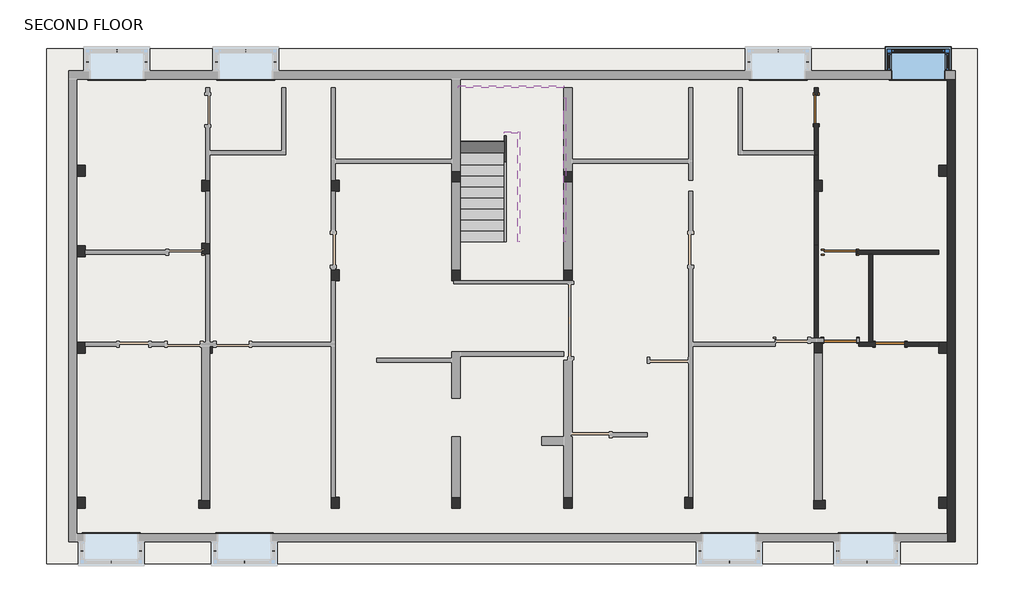
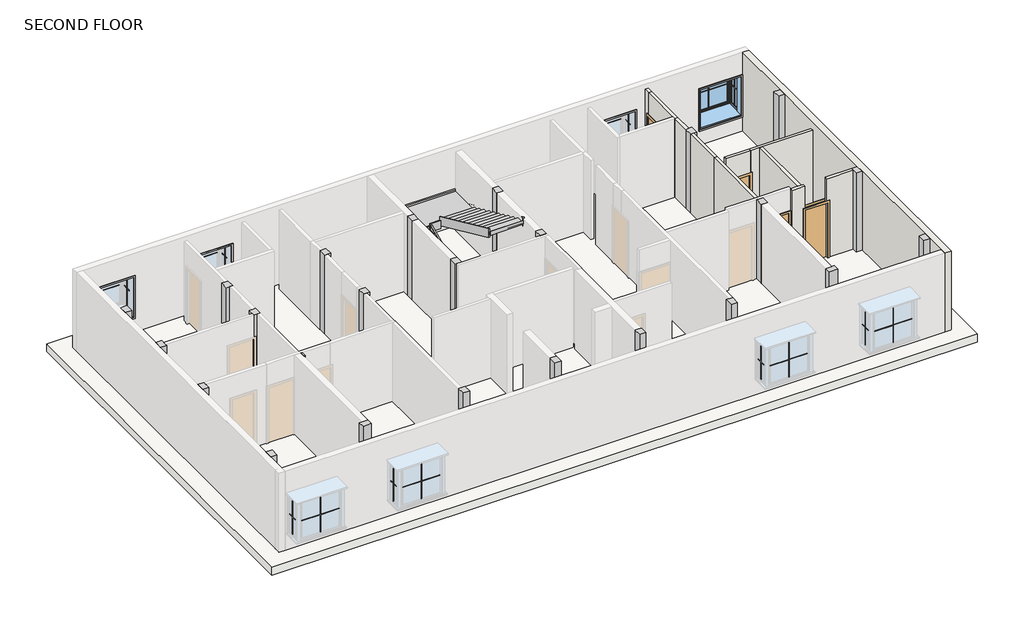
# One storey, part 2 of 2: 32 proxies, 24 columns, 11 walls, 6 members, 4 doors, 1 slab, 1 stair flight, 1 window.
"""IFC4 building model written with IfcOpenShell, lengths in millimetres."""

from ifc_helpers import new_model, si_unit, frame, origin, place, context, project, spatial, polyline, outline, extrude, faceted_brep, transform, mapped, element, save
from components import m_muntin_pattern_2x2_m_muntin_pattern_2x2_c1fd4460, m_muntin_pattern_2x2_m_muntin_pattern_2x2_777b163a, m_trim_window_interior_flat_picture_frame_44e8afef, column_216859a2, door_1991e9a2, door_a431d384, door_82def9da, m_door_single_panel_3_x7_f8176753, stair_flight_b17f4745, window_19bbd869

model = new_model("IFC4")

# Units and contexts
model_context = context("Model", 3, world=origin())
ifc_project = project(units=[si_unit("LENGTHUNIT", "METRE", prefix="MILLI")], contexts=[model_context])

# Site, building, storey
site = spatial("IfcSite", under=ifc_project)
building = spatial("IfcBuilding", under=site)
storey = spatial("IfcBuildingStorey", under=building, Name="SECOND FLOOR", Elevation=9601.2)

# Proxies
placement = place(None, origin())
m_muntin_pattern_2x2_m_muntin_pattern_2x2_shape = m_muntin_pattern_2x2_m_muntin_pattern_2x2_c1fd4460(model_context)
element("IfcBuildingElementProxy", 1, Name="M_Muntin Pattern_2x2 : M_Muntin Pattern_2x2", ObjectType="M_Muntin Pattern_2x2 : M_Muntin Pattern_2x2", at=placement, inside=storey, context=model_context, shape_type="MappedRepresentation", body=[
    mapped(m_muntin_pattern_2x2_m_muntin_pattern_2x2_shape, transform((-11500.7987957, -5499.9182661, 10321.85), x_axis=(-1.0, 0.0, 0.0), y_axis=(0.0, -1.0, 0.0), z_axis=(0.0, 0.0, 1.0))),
])
element("IfcBuildingElementProxy", 2, Name="M_Muntin Pattern_2x2 : M_Muntin Pattern_2x2", ObjectType="M_Muntin Pattern_2x2 : M_Muntin Pattern_2x2", at=placement, inside=storey, context=model_context, shape_type="MappedRepresentation", body=[
    mapped(m_muntin_pattern_2x2_m_muntin_pattern_2x2_shape, transform((-7819.250543, -5499.9182661, 10321.85), x_axis=(-1.0, 0.0, 0.0), y_axis=(0.0, -1.0, 0.0), z_axis=(0.0, 0.0, 1.0))),
])
element("IfcBuildingElementProxy", 3, Name="M_Muntin Pattern_2x2 : M_Muntin Pattern_2x2", ObjectType="M_Muntin Pattern_2x2 : M_Muntin Pattern_2x2", at=placement, inside=storey, context=model_context, shape_type="MappedRepresentation", body=[
    mapped(m_muntin_pattern_2x2_m_muntin_pattern_2x2_shape, transform((5599.7512082, -5499.9182661, 10321.85), x_axis=(-1.0, 0.0, 0.0), y_axis=(0.0, -1.0, 0.0), z_axis=(0.0, 0.0, 1.0))),
])
element("IfcBuildingElementProxy", 4, Name="M_Muntin Pattern_2x2 : M_Muntin Pattern_2x2", ObjectType="M_Muntin Pattern_2x2 : M_Muntin Pattern_2x2", at=placement, inside=storey, context=model_context, shape_type="MappedRepresentation", body=[
    mapped(m_muntin_pattern_2x2_m_muntin_pattern_2x2_shape, transform((9408.6146942, -5499.9182662, 10321.85), x_axis=(-1.0, 0.0, 0.0), y_axis=(0.0, -1.0, 0.0), z_axis=(0.0, 0.0, 1.0))),
])
element("IfcBuildingElementProxy", 5, Name="M_Muntin Pattern_2x2 : M_Muntin Pattern_2x2", ObjectType="M_Muntin Pattern_2x2 : M_Muntin Pattern_2x2", at=placement, inside=storey, context=model_context, shape_type="MappedRepresentation", body=[
    mapped(m_muntin_pattern_2x2_m_muntin_pattern_2x2_shape, transform((-11348.3987957, 8647.7317329, 10321.85), x_axis=(1.0, 0.0, 0.0), y_axis=(0.0, 1.0, 0.0), z_axis=(0.0, 0.0, 1.0))),
])
element("IfcBuildingElementProxy", 6, Name="M_Muntin Pattern_2x2 : M_Muntin Pattern_2x2", ObjectType="M_Muntin Pattern_2x2 : M_Muntin Pattern_2x2", at=placement, inside=storey, context=model_context, shape_type="MappedRepresentation", body=[
    mapped(m_muntin_pattern_2x2_m_muntin_pattern_2x2_shape, transform((-7779.6987993, 8647.7317329, 10321.85), x_axis=(1.0, 0.0, 0.0), y_axis=(0.0, 1.0, 0.0), z_axis=(0.0, 0.0, 1.0))),
])
element("IfcBuildingElementProxy", 7, Name="M_Muntin Pattern_2x2 : M_Muntin Pattern_2x2", ObjectType="M_Muntin Pattern_2x2 : M_Muntin Pattern_2x2", at=placement, inside=storey, context=model_context, shape_type="MappedRepresentation", body=[
    mapped(m_muntin_pattern_2x2_m_muntin_pattern_2x2_shape, transform((6952.301208, 8647.7317329, 10321.85), x_axis=(1.0, 0.0, 0.0), y_axis=(0.0, 1.0, 0.0), z_axis=(0.0, 0.0, 1.0))),
])
element("IfcBuildingElementProxy", 8, Name="M_Muntin Pattern_2x2 : M_Muntin Pattern_2x2", ObjectType="M_Muntin Pattern_2x2 : M_Muntin Pattern_2x2", at=placement, inside=storey, context=model_context, shape_type="MappedRepresentation", body=[
    mapped(m_muntin_pattern_2x2_m_muntin_pattern_2x2_shape, transform((10825.8012075, 8647.7317329, 10321.85), x_axis=(1.0, 0.0, 0.0), y_axis=(0.0, 1.0, 0.0), z_axis=(0.0, 0.0, 1.0))),
])
m_muntin_pattern_2x2_m_muntin_pattern_2x2_2_shape = m_muntin_pattern_2x2_m_muntin_pattern_2x2_777b163a(model_context)
element("IfcBuildingElementProxy", 9, Name="M_Muntin Pattern_2x2 : M_Muntin Pattern_2x2", ObjectType="M_Muntin Pattern_2x2 : M_Muntin Pattern_2x2", at=placement, inside=storey, context=model_context, shape_type="MappedRepresentation", body=[
    mapped(m_muntin_pattern_2x2_m_muntin_pattern_2x2_2_shape, transform((-10690.4737957, -5190.3932661, 10321.85), x_axis=(0.0, 1.0, 0.0), y_axis=(-1.0, 0.0, 0.0), z_axis=(0.0, 0.0, 1.0))),
])
element("IfcBuildingElementProxy", 10, Name="M_Muntin Pattern_2x2 : M_Muntin Pattern_2x2", ObjectType="M_Muntin Pattern_2x2 : M_Muntin Pattern_2x2", at=placement, inside=storey, context=model_context, shape_type="MappedRepresentation", body=[
    mapped(m_muntin_pattern_2x2_m_muntin_pattern_2x2_2_shape, transform((-12311.1237957, -5190.3932661, 10321.85), x_axis=(0.0, -1.0, 0.0), y_axis=(1.0, 0.0, 0.0), z_axis=(0.0, 0.0, 1.0))),
])
element("IfcBuildingElementProxy", 11, Name="M_Muntin Pattern_2x2 : M_Muntin Pattern_2x2", ObjectType="M_Muntin Pattern_2x2 : M_Muntin Pattern_2x2", at=placement, inside=storey, context=model_context, shape_type="MappedRepresentation", body=[
    mapped(m_muntin_pattern_2x2_m_muntin_pattern_2x2_2_shape, transform((-7008.925543, -5190.3932661, 10321.85), x_axis=(0.0, 1.0, 0.0), y_axis=(-1.0, 0.0, 0.0), z_axis=(0.0, 0.0, 1.0))),
])
element("IfcBuildingElementProxy", 12, Name="M_Muntin Pattern_2x2 : M_Muntin Pattern_2x2", ObjectType="M_Muntin Pattern_2x2 : M_Muntin Pattern_2x2", at=placement, inside=storey, context=model_context, shape_type="MappedRepresentation", body=[
    mapped(m_muntin_pattern_2x2_m_muntin_pattern_2x2_2_shape, transform((-8629.575543, -5190.3932661, 10321.85), x_axis=(0.0, -1.0, 0.0), y_axis=(1.0, 0.0, 0.0), z_axis=(0.0, 0.0, 1.0))),
])
element("IfcBuildingElementProxy", 13, Name="M_Muntin Pattern_2x2 : M_Muntin Pattern_2x2", ObjectType="M_Muntin Pattern_2x2 : M_Muntin Pattern_2x2", at=placement, inside=storey, context=model_context, shape_type="MappedRepresentation", body=[
    mapped(m_muntin_pattern_2x2_m_muntin_pattern_2x2_2_shape, transform((6410.0762082, -5190.3932661, 10321.85), x_axis=(0.0, 1.0, 0.0), y_axis=(-1.0, 0.0, 0.0), z_axis=(0.0, 0.0, 1.0))),
])
element("IfcBuildingElementProxy", 14, Name="M_Muntin Pattern_2x2 : M_Muntin Pattern_2x2", ObjectType="M_Muntin Pattern_2x2 : M_Muntin Pattern_2x2", at=placement, inside=storey, context=model_context, shape_type="MappedRepresentation", body=[
    mapped(m_muntin_pattern_2x2_m_muntin_pattern_2x2_2_shape, transform((4789.4262082, -5190.3932661, 10321.85), x_axis=(0.0, -1.0, 0.0), y_axis=(1.0, 0.0, 0.0), z_axis=(0.0, 0.0, 1.0))),
])
element("IfcBuildingElementProxy", 15, Name="M_Muntin Pattern_2x2 : M_Muntin Pattern_2x2", ObjectType="M_Muntin Pattern_2x2 : M_Muntin Pattern_2x2", at=placement, inside=storey, context=model_context, shape_type="MappedRepresentation", body=[
    mapped(m_muntin_pattern_2x2_m_muntin_pattern_2x2_2_shape, transform((10218.9396942, -5190.3932662, 10321.85), x_axis=(0.0, 1.0, 0.0), y_axis=(-1.0, 0.0, 0.0), z_axis=(0.0, 0.0, 1.0))),
])
element("IfcBuildingElementProxy", 16, Name="M_Muntin Pattern_2x2 : M_Muntin Pattern_2x2", ObjectType="M_Muntin Pattern_2x2 : M_Muntin Pattern_2x2", at=placement, inside=storey, context=model_context, shape_type="MappedRepresentation", body=[
    mapped(m_muntin_pattern_2x2_m_muntin_pattern_2x2_2_shape, transform((8598.2896942, -5190.3932661, 10321.85), x_axis=(0.0, -1.0, 0.0), y_axis=(1.0, 0.0, 0.0), z_axis=(0.0, 0.0, 1.0))),
])
element("IfcBuildingElementProxy", 17, Name="M_Muntin Pattern_2x2 : M_Muntin Pattern_2x2", ObjectType="M_Muntin Pattern_2x2 : M_Muntin Pattern_2x2", at=placement, inside=storey, context=model_context, shape_type="MappedRepresentation", body=[
    mapped(m_muntin_pattern_2x2_m_muntin_pattern_2x2_2_shape, transform((-12158.7237957, 8338.2067329, 10321.85), x_axis=(0.0, -1.0, 0.0), y_axis=(1.0, 0.0, 0.0), z_axis=(0.0, 0.0, 1.0))),
])
element("IfcBuildingElementProxy", 18, Name="M_Muntin Pattern_2x2 : M_Muntin Pattern_2x2", ObjectType="M_Muntin Pattern_2x2 : M_Muntin Pattern_2x2", at=placement, inside=storey, context=model_context, shape_type="MappedRepresentation", body=[
    mapped(m_muntin_pattern_2x2_m_muntin_pattern_2x2_2_shape, transform((-10538.0737957, 8338.2067329, 10321.85), x_axis=(0.0, 1.0, 0.0), y_axis=(-1.0, 0.0, 0.0), z_axis=(0.0, 0.0, 1.0))),
])
element("IfcBuildingElementProxy", 19, Name="M_Muntin Pattern_2x2 : M_Muntin Pattern_2x2", ObjectType="M_Muntin Pattern_2x2 : M_Muntin Pattern_2x2", at=placement, inside=storey, context=model_context, shape_type="MappedRepresentation", body=[
    mapped(m_muntin_pattern_2x2_m_muntin_pattern_2x2_2_shape, transform((-8590.0237993, 8338.2067329, 10321.85), x_axis=(0.0, -1.0, 0.0), y_axis=(1.0, 0.0, 0.0), z_axis=(0.0, 0.0, 1.0))),
])
element("IfcBuildingElementProxy", 20, Name="M_Muntin Pattern_2x2 : M_Muntin Pattern_2x2", ObjectType="M_Muntin Pattern_2x2 : M_Muntin Pattern_2x2", at=placement, inside=storey, context=model_context, shape_type="MappedRepresentation", body=[
    mapped(m_muntin_pattern_2x2_m_muntin_pattern_2x2_2_shape, transform((-6969.3737993, 8338.2067329, 10321.85), x_axis=(0.0, 1.0, 0.0), y_axis=(-1.0, 0.0, 0.0), z_axis=(0.0, 0.0, 1.0))),
])
element("IfcBuildingElementProxy", 21, Name="M_Muntin Pattern_2x2 : M_Muntin Pattern_2x2", ObjectType="M_Muntin Pattern_2x2 : M_Muntin Pattern_2x2", at=placement, inside=storey, context=model_context, shape_type="MappedRepresentation", body=[
    mapped(m_muntin_pattern_2x2_m_muntin_pattern_2x2_2_shape, transform((6141.976208, 8338.2067329, 10321.85), x_axis=(0.0, -1.0, 0.0), y_axis=(1.0, 0.0, 0.0), z_axis=(0.0, 0.0, 1.0))),
])
element("IfcBuildingElementProxy", 22, Name="M_Muntin Pattern_2x2 : M_Muntin Pattern_2x2", ObjectType="M_Muntin Pattern_2x2 : M_Muntin Pattern_2x2", at=placement, inside=storey, context=model_context, shape_type="MappedRepresentation", body=[
    mapped(m_muntin_pattern_2x2_m_muntin_pattern_2x2_2_shape, transform((7762.626208, 8338.2067329, 10321.85), x_axis=(0.0, 1.0, 0.0), y_axis=(-1.0, 0.0, 0.0), z_axis=(0.0, 0.0, 1.0))),
])
element("IfcBuildingElementProxy", 23, Name="M_Muntin Pattern_2x2 : M_Muntin Pattern_2x2", ObjectType="M_Muntin Pattern_2x2 : M_Muntin Pattern_2x2", at=placement, inside=storey, context=model_context, shape_type="MappedRepresentation", body=[
    mapped(m_muntin_pattern_2x2_m_muntin_pattern_2x2_2_shape, transform((10015.4762075, 8338.2067329, 10321.85), x_axis=(0.0, -1.0, 0.0), y_axis=(1.0, 0.0, 0.0), z_axis=(0.0, 0.0, 1.0))),
])
element("IfcBuildingElementProxy", 24, Name="M_Muntin Pattern_2x2 : M_Muntin Pattern_2x2", ObjectType="M_Muntin Pattern_2x2 : M_Muntin Pattern_2x2", at=placement, inside=storey, context=model_context, shape_type="MappedRepresentation", body=[
    mapped(m_muntin_pattern_2x2_m_muntin_pattern_2x2_2_shape, transform((11636.1262075, 8338.2067329, 10321.85), x_axis=(0.0, 1.0, 0.0), y_axis=(-1.0, 0.0, 0.0), z_axis=(0.0, 0.0, 1.0))),
])
m_trim_window_interior_flat_picture_frame_shape = m_trim_window_interior_flat_picture_frame_44e8afef(model_context)
element("IfcBuildingElementProxy", 25, Name="M_Trim-Window-Interior-Flat : Picture Frame", ObjectType="M_Trim-Window-Interior-Flat : Picture Frame", at=placement, inside=storey, context=model_context, shape_type="MappedRepresentation", body=[
    mapped(m_trim_window_interior_flat_picture_frame_shape, transform((-11500.7987957, -4712.5932661, 11752.0), x_axis=(-1.0, 0.0, 0.0), y_axis=(0.0, 0.0, 1.0), z_axis=(0.0, 1.0, 0.0))),
])
element("IfcBuildingElementProxy", 26, Name="M_Trim-Window-Interior-Flat : Picture Frame", ObjectType="M_Trim-Window-Interior-Flat : Picture Frame", at=placement, inside=storey, context=model_context, shape_type="MappedRepresentation", body=[
    mapped(m_trim_window_interior_flat_picture_frame_shape, transform((-7819.250543, -4712.5932661, 11752.0), x_axis=(-1.0, 0.0, 0.0), y_axis=(0.0, 0.0, 1.0), z_axis=(0.0, 1.0, 0.0))),
])
element("IfcBuildingElementProxy", 27, Name="M_Trim-Window-Interior-Flat : Picture Frame", ObjectType="M_Trim-Window-Interior-Flat : Picture Frame", at=placement, inside=storey, context=model_context, shape_type="MappedRepresentation", body=[
    mapped(m_trim_window_interior_flat_picture_frame_shape, transform((5599.7512082, -4712.5932661, 11752.0), x_axis=(-1.0, 0.0, 0.0), y_axis=(0.0, 0.0, 1.0), z_axis=(0.0, 1.0, 0.0))),
])
element("IfcBuildingElementProxy", 28, Name="M_Trim-Window-Interior-Flat : Picture Frame", ObjectType="M_Trim-Window-Interior-Flat : Picture Frame", at=placement, inside=storey, context=model_context, shape_type="MappedRepresentation", body=[
    mapped(m_trim_window_interior_flat_picture_frame_shape, transform((9408.6146942, -4712.5932661, 11752.0), x_axis=(-1.0, 0.0, 0.0), y_axis=(0.0, 0.0, 1.0), z_axis=(0.0, 1.0, 0.0))),
])
element("IfcBuildingElementProxy", 29, Name="M_Trim-Window-Interior-Flat : Picture Frame", ObjectType="M_Trim-Window-Interior-Flat : Picture Frame", at=placement, inside=storey, context=model_context, shape_type="MappedRepresentation", body=[
    mapped(m_trim_window_interior_flat_picture_frame_shape, transform((-11348.3987957, 7860.4067329, 11752.0), x_axis=(1.0, 0.0, 0.0), y_axis=(0.0, 0.0, 1.0), z_axis=(0.0, -1.0, 0.0))),
])
element("IfcBuildingElementProxy", 30, Name="M_Trim-Window-Interior-Flat : Picture Frame", ObjectType="M_Trim-Window-Interior-Flat : Picture Frame", at=placement, inside=storey, context=model_context, shape_type="MappedRepresentation", body=[
    mapped(m_trim_window_interior_flat_picture_frame_shape, transform((-7779.6987993, 7860.4067329, 11752.0), x_axis=(1.0, 0.0, 0.0), y_axis=(0.0, 0.0, 1.0), z_axis=(0.0, -1.0, 0.0))),
])
element("IfcBuildingElementProxy", 31, Name="M_Trim-Window-Interior-Flat : Picture Frame", ObjectType="M_Trim-Window-Interior-Flat : Picture Frame", at=placement, inside=storey, context=model_context, shape_type="MappedRepresentation", body=[
    mapped(m_trim_window_interior_flat_picture_frame_shape, transform((6952.301208, 7860.4067329, 11752.0), x_axis=(1.0, 0.0, 0.0), y_axis=(0.0, 0.0, 1.0), z_axis=(0.0, -1.0, 0.0))),
])
element("IfcBuildingElementProxy", 32, Name="M_Trim-Window-Interior-Flat : Picture Frame", ObjectType="M_Trim-Window-Interior-Flat : Picture Frame", at=placement, inside=storey, context=model_context, shape_type="MappedRepresentation", body=[
    mapped(m_trim_window_interior_flat_picture_frame_shape, transform((10825.8012075, 7860.4067329, 11752.0), x_axis=(1.0, 0.0, 0.0), y_axis=(0.0, 0.0, 1.0), z_axis=(0.0, -1.0, 0.0))),
])

# Columns
element("IfcColumn", 33, ObjectType="Rectangular Column : 1'X 9\"", at=placement, inside=storey, context=model_context, shape_type="SweptSolid", body=[
    extrude(outline(polyline([(-12224.6987957, -3709.2932671), (-12224.6987957, -4014.0932671), (-12453.2987957, -4014.0932671), (-12453.2987957, -3709.2932671), (-12224.6987957, -3709.2932671)])), frame((0.0, 0.0, 9601.2), z_axis=(0.0, 0.0, 1.0), x_axis=(1.0, 0.0, 0.0)), (0.0, 0.0, 1.0), 3048.0),
])
element("IfcColumn", 34, ObjectType="Rectangular Column : 1'X 9\"", at=placement, inside=storey, context=model_context, shape_type="SweptSolid", body=[
    extrude(outline(polyline([(-12224.6987957, 583.3067334), (-12224.6987957, 278.5067334), (-12453.2987957, 278.5067334), (-12453.2987957, 583.3067334), (-12224.6987957, 583.3067334)])), frame((0.0, 0.0, 9601.2), z_axis=(0.0, 0.0, 1.0), x_axis=(1.0, 0.0, 0.0)), (0.0, 0.0, 1.0), 3048.0),
])
element("IfcColumn", 35, ObjectType="Rectangular Column : 1'X 9\"", at=placement, inside=storey, context=model_context, shape_type="SweptSolid", body=[
    extrude(outline(polyline([(-12224.6987957, 3256.6567332), (-12224.6987957, 2951.8567332), (-12453.2987957, 2951.8567332), (-12453.2987957, 3256.6567332), (-12224.6987957, 3256.6567332)])), frame((0.0, 0.0, 9601.2), z_axis=(0.0, 0.0, 1.0), x_axis=(1.0, 0.0, 0.0)), (0.0, 0.0, 1.0), 3048.0),
])
element("IfcColumn", 36, ObjectType="Rectangular Column : 1'X 9\"", at=placement, inside=storey, context=model_context, shape_type="Brep", body=[
    faceted_brep([(-8770.2987992, 5066.406733, 9601.2), (-8770.2987992, 4761.606733, 9601.2), (-8884.5987992, 4761.606733, 9601.2), (-8998.8987992, 4761.606733, 9601.2), (-8998.8987992, 5066.406733, 9601.2), (-8884.5987992, 5066.406733, 9601.2), (-8770.2987992, 5066.406733, 12649.2), (-8770.2987992, 4761.606733, 12649.2), (-8884.5987992, 4761.606733, 12649.2), (-8998.8987992, 4761.606733, 12649.2), (-8998.8987992, 5066.406733, 12649.2), (-8884.5987992, 5066.406733, 12649.2)], [[[0, 1, 2, 3, 4, 5]], [[6, 7, 1, 0]], [[7, 8, 9, 3, 2, 1]], [[9, 10, 4, 3]], [[10, 11, 6, 0, 5, 4]], [[6, 11, 10, 9, 8, 7]]]),
])
element("IfcColumn", 37, ObjectType="Rectangular Column : 1'X 9\"", at=placement, inside=storey, context=model_context, shape_type="Brep", body=[
    faceted_brep([(-8770.2987992, 3326.5067332, 9601.2), (-8770.2987992, 3021.7067332, 9601.2), (-8884.598796, 3021.7067332, 9601.2), (-8998.8987992, 3021.7067332, 9601.2), (-8998.8987992, 3326.5067332, 9601.2), (-8884.5987992, 3326.5067332, 9601.2), (-8770.2987992, 3326.5067332, 12649.2), (-8770.2987992, 3021.7067332, 12649.2), (-8884.598796, 3021.7067332, 12649.2), (-8998.8987992, 3021.7067332, 12649.2), (-8998.8987992, 3326.5067332, 12649.2), (-8884.5987992, 3326.5067332, 12649.2)], [[[0, 1, 2, 3, 4, 5]], [[6, 7, 1, 0]], [[7, 8, 9, 3, 2, 1]], [[9, 10, 4, 3]], [[10, 11, 6, 0, 5, 4]], [[6, 11, 10, 9, 8, 7]]]),
])
element("IfcColumn", 38, ObjectType="Rectangular Column : 1'X 9\"", at=placement, inside=storey, context=model_context, shape_type="SweptSolid", body=[
    extrude(outline(polyline([(-8713.148796, 278.5067334), (-8771.750543, 278.5067334), (-8771.750543, 469.0067334), (-8713.148796, 469.0067334), (-8713.148796, 278.5067334)])), frame((0.0, 0.0, 9601.2), z_axis=(0.0, 0.0, 1.0), x_axis=(1.0, 0.0, 0.0)), (0.0, 0.0, 1.0), 3048.0),
])
element("IfcColumn", 39, ObjectType="Rectangular Column : 1'X 9\"", at=placement, inside=storey, context=model_context, shape_type="Brep", body=[
    faceted_brep([(-5188.8987995, 5066.406733, 9601.2), (-5188.8987995, 4761.606733, 9601.2), (-5303.1987995, 4761.606733, 9601.2), (-5417.4987995, 4761.606733, 9601.2), (-5417.4987995, 5066.406733, 9601.2), (-5303.1987995, 5066.406733, 9601.2), (-5188.8987995, 5066.406733, 12649.2), (-5188.8987995, 4761.606733, 12649.2), (-5303.1987995, 4761.606733, 12649.2), (-5417.4987995, 4761.606733, 12649.2), (-5417.4987995, 5066.406733, 12649.2), (-5303.1987995, 5066.406733, 12649.2)], [[[0, 1, 2, 3, 4, 5]], [[6, 7, 1, 0]], [[7, 8, 9, 3, 2, 1]], [[9, 10, 4, 3]], [[10, 11, 6, 0, 5, 4]], [[6, 11, 10, 9, 8, 7]]]),
])
element("IfcColumn", 40, ObjectType="Rectangular Column : 1'X 9\"", at=placement, inside=storey, context=model_context, shape_type="Brep", body=[
    faceted_brep([(-5188.8987995, 2589.9067802, 9601.2), (-5188.8987995, 2285.1067802, 9601.2), (-5303.1987995, 2285.1067802, 9601.2), (-5417.4987995, 2285.1067802, 9601.2), (-5417.4987995, 2589.9067802, 9601.2), (-5303.1987995, 2589.9067802, 9601.2), (-5188.8987995, 2589.9067802, 12649.2), (-5188.8987995, 2285.1067802, 12649.2), (-5303.1987995, 2285.1067802, 12649.2), (-5417.4987995, 2285.1067802, 12649.2), (-5417.4987995, 2589.9067802, 12649.2), (-5303.1987995, 2589.9067802, 12649.2)], [[[0, 1, 2, 3, 4, 5]], [[6, 7, 1, 0]], [[7, 8, 9, 3, 2, 1]], [[9, 10, 4, 3]], [[10, 11, 6, 0, 5, 4]], [[6, 11, 10, 9, 8, 7]]]),
])
element("IfcColumn", 41, ObjectType="Rectangular Column : 1'X 9\"", at=placement, inside=storey, context=model_context, shape_type="Brep", body=[
    faceted_brep([(-5188.8987963, -3709.2932193, 9601.2), (-5188.8987963, -4014.0932193, 9601.2), (-5417.4987963, -4014.0932193, 9601.2), (-5417.4987963, -3709.2932193, 9601.2), (-5303.1987995, -3709.2932193, 9601.2), (-5188.8987963, -3709.2932193, 12649.2), (-5188.8987963, -4014.0932193, 12649.2), (-5417.4987963, -4014.0932193, 12649.2), (-5417.4987963, -3709.2932193, 12649.2), (-5303.1987995, -3709.2932193, 12649.2)], [[[0, 1, 2, 3, 4]], [[5, 6, 1, 0]], [[6, 7, 2, 1]], [[7, 8, 3, 2]], [[8, 9, 5, 0, 4, 3]], [[5, 9, 8, 7, 6]]]),
])
element("IfcColumn", 42, ObjectType="Rectangular Column : 1'X 9\"", at=placement, inside=storey, context=model_context, shape_type="SweptSolid", body=[
    extrude(outline(polyline([(1250.0012085, -3709.2932193), (1250.0012085, -4014.0932193), (1021.4012085, -4014.0932193), (1021.4012085, -3709.2932193), (1250.0012085, -3709.2932193)])), frame((0.0, 0.0, 9601.2), z_axis=(0.0, 0.0, 1.0), x_axis=(1.0, 0.0, 0.0)), (0.0, 0.0, 1.0), 3048.0),
])
element("IfcColumn", 43, ObjectType="Rectangular Column : 1'X 9\"", at=placement, inside=storey, context=model_context, shape_type="Brep", body=[
    faceted_brep([(4590.1012082, -3709.2932193, 9601.2), (4590.1012082, -4014.0932193, 9601.2), (4361.5012082, -4014.0932193, 9601.2), (4361.5012082, -3709.2932193, 9601.2), (4475.8012082, -3709.2932193, 9601.2), (4590.1012082, -3709.2932193, 12649.2), (4590.1012082, -4014.0932193, 12649.2), (4361.5012082, -4014.0932193, 12649.2), (4361.5012082, -3709.2932193, 12649.2), (4475.8012082, -3709.2932193, 12649.2)], [[[0, 1, 2, 3, 4]], [[5, 6, 1, 0]], [[6, 7, 2, 1]], [[7, 8, 3, 2]], [[8, 9, 5, 0, 4, 3]], [[5, 9, 8, 7, 6]]]),
])
element("IfcColumn", 44, ObjectType="Rectangular Column : 1'X 9\"", at=placement, inside=storey, context=model_context, shape_type="SweptSolid", body=[
    extrude(outline(polyline([(11625.9012075, -3709.2932671), (11625.9012075, -4014.0932671), (11397.3012075, -4014.0932671), (11397.3012075, -3709.2932671), (11625.9012075, -3709.2932671)])), frame((0.0, 0.0, 9601.2), z_axis=(0.0, 0.0, 1.0), x_axis=(1.0, 0.0, 0.0)), (0.0, 0.0, 1.0), 3048.0),
])
element("IfcColumn", 45, ObjectType="Rectangular Column : 1'X 9\"", at=placement, inside=storey, context=model_context, shape_type="Brep", body=[
    faceted_brep([(11625.9012075, 583.3067295, 9601.2), (11625.9012075, 278.5067295, 9601.2), (11397.3012075, 278.5067295, 9601.2), (11397.3012075, 469.0067295, 9601.2), (11397.3012075, 583.3067295, 9601.2), (11625.9012075, 583.3067295, 12649.2), (11625.9012075, 278.5067295, 12649.2), (11397.3012075, 278.5067295, 12649.2), (11397.3012075, 469.0067295, 12649.2), (11397.3012075, 583.3067295, 12649.2)], [[[0, 1, 2, 3, 4]], [[5, 6, 1, 0]], [[6, 7, 2, 1]], [[7, 8, 9, 4, 3, 2]], [[9, 5, 0, 4]], [[5, 9, 8, 7, 6]]]),
])
element("IfcColumn", 46, ObjectType="Rectangular Column : 1'X 9\"", at=placement, inside=storey, context=model_context, shape_type="SweptSolid", body=[
    extrude(outline(polyline([(11625.9012075, 5479.1567329), (11625.9012075, 5174.3567329), (11397.3012075, 5174.3567329), (11397.3012075, 5479.1567329), (11625.9012075, 5479.1567329)])), frame((0.0, 0.0, 9601.2), z_axis=(0.0, 0.0, 1.0), x_axis=(1.0, 0.0, 0.0)), (0.0, 0.0, 1.0), 3048.0),
])
element("IfcColumn", 47, ObjectType="Rectangular Column : 1'X 9\"", at=placement, inside=storey, context=model_context, shape_type="Brep", body=[
    faceted_brep([(8172.5040565, 5065.4824989, 9601.2), (8172.5040565, 4760.6824989, 9601.2), (8057.2012047, 4760.6824989, 9601.2), (7943.9040565, 4760.6824989, 9601.2), (7943.9040565, 5065.4824989, 9601.2), (8058.2040565, 5065.4824989, 9601.2), (8172.5040565, 5065.4824989, 12649.2), (8172.5040565, 4760.6824989, 12649.2), (8057.2012047, 4760.6824989, 12649.2), (7943.9040565, 4760.6824989, 12649.2), (7943.9040565, 5065.4824989, 12649.2), (8058.2040565, 5065.4824989, 12649.2)], [[[0, 1, 2, 3, 4, 5]], [[6, 7, 1, 0]], [[7, 8, 9, 3, 2, 1]], [[9, 10, 4, 3]], [[10, 11, 6, 0, 5, 4]], [[6, 11, 10, 9, 8, 7]]]),
])
element("IfcColumn", 48, ObjectType="Rectangular Column : 1'X 9\"", at=placement, inside=storey, context=model_context, shape_type="Brep", body=[
    faceted_brep([(8171.5012047, 583.3067334, 9601.2), (8171.5012047, 278.5067334, 9601.2), (7942.9012047, 278.5067334, 9601.2), (7942.9012047, 583.3067334, 9601.2), (8000.0512079, 583.3067334, 9601.2), (8171.5012047, 583.3067334, 12649.2), (8171.5012047, 278.5067334, 12649.2), (7942.9012047, 278.5067334, 12649.2), (7942.9012047, 583.3067334, 12649.2), (8000.0512079, 583.3067334, 12649.2)], [[[0, 1, 2, 3, 4]], [[5, 6, 1, 0]], [[6, 7, 2, 1]], [[7, 8, 3, 2]], [[8, 9, 5, 0, 4, 3]], [[5, 9, 8, 7, 6]]]),
])
element("IfcColumn", 49, ObjectType="Rectangular Column : 1'X 9\"", at=placement, inside=storey, context=model_context, shape_type="Brep", body=[
    faceted_brep([(-9076.550543, -3785.4932196, 9601.2), (-9000.350543, -3785.4932196, 9601.2), (-8771.750543, -3785.4932196, 9601.2), (-8771.750543, -4014.0932196, 9601.2), (-9076.550543, -4014.0932196, 9601.2), (-9076.550543, -3785.4932196, 12649.2), (-9000.350543, -3785.4932196, 12649.2), (-8771.750543, -3785.4932196, 12649.2), (-8771.750543, -4014.0932196, 12649.2), (-9076.550543, -4014.0932196, 12649.2)], [[[0, 1, 2, 3, 4]], [[5, 6, 7, 2, 1, 0]], [[7, 8, 3, 2]], [[8, 9, 4, 3]], [[9, 5, 0, 4]], [[5, 9, 8, 7, 6]]]),
])
element("IfcColumn", 50, ObjectType="Rectangular Column : 1'X 9\"", at=placement, inside=storey, context=model_context, shape_type="SweptSolid", body=[
    extrude(outline(polyline([(-12453.2987957, 5174.3567339), (-12453.2987957, 5479.1567339), (-12224.6987957, 5479.1567339), (-12224.6987957, 5174.3567339), (-12453.2987957, 5174.3567339)])), frame((0.0, 0.0, 9601.2), z_axis=(0.0, 0.0, 1.0), x_axis=(1.0, 0.0, 0.0)), (0.0, 0.0, 1.0), 3048.0),
])
element("IfcColumn", 51, ObjectType="Rectangular Column : 1'X 9\"", at=placement, inside=storey, context=model_context, shape_type="SweptSolid", body=[
    extrude(outline(polyline([(-1845.5417538, 5320.4067329), (-1845.5417538, 5015.6067329), (-2074.1417538, 5015.6067329), (-2074.1417538, 5320.4067329), (-1845.5417538, 5320.4067329)])), frame((0.0, 0.0, 9601.2), z_axis=(0.0, 0.0, 1.0), x_axis=(1.0, 0.0, 0.0)), (0.0, 0.0, 1.0), 3048.0),
])
element("IfcColumn", 52, ObjectType="Rectangular Column : 1'X 9\"", at=placement, inside=storey, context=model_context, shape_type="SweptSolid", body=[
    extrude(outline(polyline([(1250.0012085, 5320.4067329), (1250.0012085, 5015.6067329), (1021.4012085, 5015.6067329), (1021.4012085, 5320.4067329), (1250.0012085, 5320.4067329)])), frame((0.0, 0.0, 9601.2), z_axis=(0.0, 0.0, 1.0), x_axis=(1.0, 0.0, 0.0)), (0.0, 0.0, 1.0), 3048.0),
])
element("IfcColumn", 53, ObjectType="Rectangular Column : 1'X 9\"", at=placement, inside=storey, context=model_context, shape_type="Brep", body=[
    faceted_brep([(-1845.5417538, 2589.906774, 9601.2), (-1845.5417538, 2285.106774, 9601.2), (-2020.2487998, 2285.106774, 9601.2), (-2074.1417538, 2285.106774, 9601.2), (-2074.1417538, 2589.906774, 9601.2), (-1845.5417538, 2589.906774, 12649.2), (-1845.5417538, 2285.106774, 12649.2), (-2020.2487998, 2285.106774, 12649.2), (-2074.1417538, 2285.106774, 12649.2), (-2074.1417538, 2589.906774, 12649.2)], [[[0, 1, 2, 3, 4]], [[5, 6, 1, 0]], [[6, 7, 8, 3, 2, 1]], [[8, 9, 4, 3]], [[9, 5, 0, 4]], [[5, 9, 8, 7, 6]]]),
])
element("IfcColumn", 54, ObjectType="Rectangular Column : 1'X 9\"", at=placement, inside=storey, context=model_context, shape_type="Brep", body=[
    faceted_brep([(1253.2582462, 2589.9067742, 9601.2), (1253.2582462, 2285.1067742, 9601.2), (1024.6582462, 2285.1067742, 9601.2), (1024.6582462, 2589.9067742, 9601.2), (1250.0012085, 2589.9067742, 9601.2), (1253.2582462, 2589.9067742, 12649.2), (1253.2582462, 2285.1067742, 12649.2), (1024.6582462, 2285.1067742, 12649.2), (1024.6582462, 2589.9067742, 12649.2), (1250.0012085, 2589.9067742, 12649.2)], [[[0, 1, 2, 3, 4]], [[5, 6, 1, 0]], [[6, 7, 2, 1]], [[7, 8, 3, 2]], [[8, 9, 5, 0, 4, 3]], [[5, 9, 8, 7, 6]]]),
])
element("IfcColumn", 55, ObjectType="Rectangular Column : 1'X 9\"", at=placement, inside=storey, context=model_context, shape_type="SweptSolid", body=[
    extrude(outline(polyline([(-1848.7987998, -3709.2932663), (-1848.7987998, -4014.0932663), (-2077.3987998, -4014.0932663), (-2077.3987998, -3709.2932663), (-1848.7987998, -3709.2932663)])), frame((0.0, 0.0, 9601.2), z_axis=(0.0, 0.0, 1.0), x_axis=(1.0, 0.0, 0.0)), (0.0, 0.0, 1.0), 3048.0),
])
column_shape = column_216859a2(model_context)
element("IfcColumn", 56, ObjectType="Rectangular Column : 1'X 9\"", at=placement, inside=storey, context=model_context, shape_type="MappedRepresentation", body=[
    mapped(column_shape, transform((8094.1646942, -3901.6914801, 0.0), x_axis=(0.0, 1.0, 0.0), y_axis=(-1.0, 0.0, 0.0), z_axis=(0.0, 0.0, 1.0))),
])

# Doors
door_shape = door_1991e9a2(model_context)
element("IfcDoor", 57, ObjectType="M_Door-Single-Panel : 2'11\"X7' 3", at=placement, inside=storey, context=model_context, shape_type="MappedRepresentation", body=[
    mapped(door_shape, transform((8664.274939, 3078.8567332, 9601.2), x_axis=(-1.0, 0.0, 0.0), y_axis=(0.0, -1.0, 0.0), z_axis=(0.0, 0.0, 1.0))),
])
door_2_shape = door_a431d384(model_context)
element("IfcDoor", 58, ObjectType="M_Door-Single-Panel : 2'7\"X7' 2", at=placement, inside=storey, context=model_context, shape_type="MappedRepresentation", body=[
    mapped(door_2_shape, transform((8000.0512079, 7021.3751452, 9601.2), x_axis=(0.0, 1.0, 0.0), y_axis=(-1.0, 0.0, 0.0), z_axis=(0.0, 0.0, 1.0))),
])
door_3_shape = door_82def9da(model_context)
element("IfcDoor", 59, ObjectType="M_Door-Single-Panel : 2'8\"X7'", at=placement, inside=storey, context=model_context, shape_type="MappedRepresentation", body=[
    mapped(door_3_shape, transform((10046.0486694, 526.1567295, 9601.2), x_axis=(-1.0, 0.0, 0.0), y_axis=(0.0, -1.0, 0.0), z_axis=(0.0, 0.0, 1.0))),
])
m_door_single_panel_3_x7_shape = m_door_single_panel_3_x7_f8176753(model_context)
element("IfcDoor", 60, ObjectType="M_Door-Single-Panel : 3'X7'", at=placement, inside=storey, context=model_context, shape_type="MappedRepresentation", body=[
    mapped(m_door_single_panel_3_x7_shape, transform((8666.8012079, 640.4567334, 9601.2), x_axis=(-1.0, 0.0, 0.0), y_axis=(0.0, -1.0, 0.0), z_axis=(0.0, 0.0, 1.0))),
])

# Members
element("IfcMember", 61, ObjectType="Stringer - 2\" Width", at=placement, inside=storey, context=model_context, shape_type="SweptSolid", body=[
    extrude(outline(polyline([(3364.6067329, 9601.2), (3364.6067329, 9801.0262721), (6445.4289342, 11201.4), (7182.0114168, 11201.4), (3661.5714168, 9601.2), (3364.6067329, 9601.2)])), frame((-1896.3417538, 0.0, 0.0), z_axis=(1.0, 0.0, 0.0), x_axis=(0.0, 1.0, 0.0)), (0.0, 0.0, 1.0), 50.8),
])
element("IfcMember", 62, ObjectType="Stringer - 2\" Width", at=placement, inside=storey, context=model_context, shape_type="SweptSolid", body=[
    extrude(outline(polyline([(-1896.3417538, 7631.8067329), (-1896.3417538, 7682.6067329), (1021.4012085, 7682.6067329), (1021.4012085, 7631.8067329), (-1896.3417538, 7631.8067329)])), frame((0.0, 0.0, 10896.6), z_axis=(0.0, 0.0, 1.0), x_axis=(1.0, 0.0, 0.0)), (0.0, 0.0, 1.0), 304.8),
])
element("IfcMember", 63, ObjectType="Stringer - 2\" Width", at=placement, inside=storey, context=model_context, shape_type="SweptSolid", body=[
    extrude(outline(polyline([(6618.562049, 10896.6), (3364.6067329, 12375.6705982), (3364.6067329, 12710.4808176), (7355.1445316, 10896.6), (6618.562049, 10896.6)])), frame((1021.4012085, 0.0, 0.0), z_axis=(1.0, 0.0, 0.0), x_axis=(0.0, 1.0, 0.0)), (0.0, 0.0, 1.0), 50.8),
])
element("IfcMember", 64, ObjectType="Stringer - 2\" Width", at=placement, inside=storey, context=model_context, shape_type="SweptSolid", body=[
    extrude(outline(polyline([(3364.6067329, 9601.2), (3364.6067329, 9801.0262721), (6361.8067329, 11163.3899085), (6361.8067329, 10828.5796892), (3661.5714168, 9601.2), (3364.6067329, 9601.2)])), frame((-629.5987998, 0.0, 0.0), z_axis=(1.0, 0.0, 0.0), x_axis=(0.0, 1.0, 0.0)), (0.0, 0.0, 1.0), 50.8),
])
element("IfcMember", 65, ObjectType="Stringer - 2\" Width", at=placement, inside=storey, context=model_context, shape_type="SweptSolid", body=[
    extrude(outline(polyline([(-629.5987998, 6361.8067329), (-629.5987998, 6412.6067329), (-248.5987915, 6412.6067329), (-248.5987915, 6361.8067329), (-629.5987998, 6361.8067329)])), frame((0.0, 0.0, 10896.6), z_axis=(0.0, 0.0, 1.0), x_axis=(1.0, 0.0, 0.0)), (0.0, 0.0, 1.0), 304.8),
])
element("IfcMember", 66, ObjectType="Stringer - 2\" Width", at=placement, inside=storey, context=model_context, shape_type="SweptSolid", body=[
    extrude(outline(polyline([(6412.6067329, 11325.0262721), (6412.6067329, 10990.2160528), (3364.6067329, 12375.6705982), (3364.6067329, 12710.4808176), (6412.6067329, 11325.0262721)])), frame((-248.5987915, 0.0, 0.0), z_axis=(1.0, 0.0, 0.0), x_axis=(0.0, 1.0, 0.0)), (0.0, 0.0, 1.0), 50.8),
])

# Slab
element("IfcSlab", 67, ObjectType="Generic - 12\"", at=placement, inside=storey, context=model_context, shape_type="SweptSolid", body=[
    extrude(outline(polyline([(12464.1012075, 8698.6067329), (12464.1012075, -5550.7932662), (-13291.4987957, -5550.7932662), (-13291.4987957, 8698.6067329), (12464.1012075, 8698.6067329)])), frame((0.0, 0.0, 9296.4), z_axis=(0.0, 0.0, 1.0), x_axis=(1.0, 0.0, 0.0)), (0.0, 0.0, 1.0), 304.8),
])

# Stair flight
stair_flight_shape = stair_flight_b17f4745(model_context)
element("IfcStairFlight", 68, ObjectType="2\" Tread 1\" Nosing 1/4\" Riser", at=placement, inside=storey, context=model_context, shape_type="MappedRepresentation", body=[
    mapped(stair_flight_shape, transform((0.0, 0.0, 0.0), x_axis=(1.0, 0.0, 0.0), y_axis=(0.0, 1.0, 0.0), z_axis=(0.0, 0.0, 1.0))),
])

# Walls
element("IfcWall", 69, ObjectType="4.5\"", at=placement, inside=storey, context=model_context, shape_type="SweptSolid", body=[
    extrude(outline(polyline([(9601.2, 9131.6486701), (12649.2, 9131.6486701), (12649.2, 8245.174939), (11734.8, 8245.174939), (11734.8, 9108.774939), (9601.2, 9108.774939), (9601.2, 9131.6486701)])), frame((0.0, 3021.7067332, 0.0), z_axis=(0.0, 1.0, 0.0), x_axis=(0.0, 0.0, 1.0)), (0.0, 0.0, 1.0), 114.3),
])
element("IfcWall", 70, ObjectType="4.5\"", at=placement, inside=storey, context=model_context, shape_type="Brep", body=[
    faceted_brep([(7942.9012079, 5764.9067329, 12649.2), (7942.9012079, 5879.2067329, 12649.2), (7942.9012079, 7415.0751452, 12649.2), (7942.9012079, 7415.0751452, 11734.8), (7942.9012079, 6627.6751452, 11734.8), (7942.9012079, 6627.6751452, 9601.2), (7942.9012079, 5879.2067329, 9601.2), (7942.9012079, 5764.9067329, 9601.2), (8057.2012079, 7415.0751452, 12649.2), (8057.2012079, 5764.9067329, 12649.2), (8057.2012079, 5764.9067329, 9601.2), (8057.2012079, 6627.6751452, 9601.2), (8057.2012079, 6627.6751452, 11734.8), (8057.2012079, 7415.0751452, 11734.8)], [[[0, 1, 2, 3, 4, 5, 6, 7]], [[8, 9, 10, 11, 12, 13]], [[10, 7, 6, 5, 11]], [[2, 1, 0, 9, 8]], [[2, 8, 13, 3]], [[12, 4, 3, 13]], [[4, 12, 11, 5]], [[0, 7, 10, 9]]]),
])
element("IfcWall", 71, ObjectType="4.5\"", at=placement, inside=storey, context=model_context, shape_type="Brep", body=[
    faceted_brep([(7942.9012079, 7631.8067329, 9601.2), (7942.9012079, 7415.0751452, 9601.2), (7942.9012079, 7415.0751452, 11734.8), (7942.9012079, 7415.0751452, 12649.2), (7942.9012079, 7631.8067329, 12649.2), (8057.2012079, 7631.8067329, 9601.2), (8057.2012079, 7631.8067329, 12649.2), (8057.2012079, 7415.0751452, 12649.2), (8057.2012079, 7415.0751452, 11734.8), (8057.2012079, 7415.0751452, 9601.2)], [[[0, 1, 2, 3, 4]], [[5, 6, 7, 8, 9]], [[1, 0, 5, 9]], [[3, 2, 1, 9, 8, 7]], [[4, 3, 7, 6]], [[0, 4, 6, 5]]]),
])
element("IfcWall", 72, ObjectType="4.5\"", at=placement, inside=storey, context=model_context, shape_type="Brep", body=[
    faceted_brep([(8057.2012047, 3270.1432417, 9601.2), (8057.2012047, 4760.6824989, 9601.2), (8057.2012047, 4760.6824989, 12649.2), (8057.2012047, 3270.1432417, 12649.2), (7942.9012047, 3270.1432417, 9601.2), (7942.9012047, 3270.1432417, 12649.2), (7942.9012047, 4760.6824989, 12649.2), (7942.9012047, 4760.6824989, 9601.2), (7943.9040565, 4760.6824989, 9601.2), (7943.9040565, 4760.6824989, 12649.2)], [[[0, 1, 2, 3]], [[4, 5, 6, 7]], [[1, 0, 4, 7, 8]], [[2, 1, 8, 7, 6, 9]], [[3, 2, 9, 6, 5]], [[0, 3, 5, 4]]]),
])
element("IfcWall", 73, ObjectType="4.5\"", at=placement, inside=storey, context=model_context, shape_type="Brep", body=[
    faceted_brep([(7942.9012079, 3270.1432417, 9601.2), (7942.9012079, 697.6067334, 9601.2), (7942.9012079, 697.6067334, 12649.2), (7942.9012079, 3270.1432417, 12649.2), (8057.2012079, 3270.1432417, 9601.2), (8057.2012079, 3270.1432417, 12649.2), (8057.2012079, 697.6067334, 12649.2), (8057.2012079, 697.6067334, 9601.2), (8000.0512079, 697.6067334, 9601.2), (8000.0512079, 697.6067334, 12649.2)], [[[0, 1, 2, 3]], [[4, 5, 6, 7]], [[1, 0, 4, 7, 8]], [[3, 2, 9, 6, 5]], [[0, 3, 5, 4]], [[2, 1, 8, 7, 6, 9]]]),
])
element("IfcWall", 74, ObjectType="4.5\"", at=placement, inside=storey, context=model_context, shape_type="SweptSolid", body=[
    extrude(outline(polyline([(8058.2040565, 5763.9824989), (8058.2040565, 5065.4824989), (7943.9040565, 5065.4824989), (7943.9040565, 5763.9824989), (8058.2040565, 5763.9824989)])), frame((0.0, 0.0, 9601.2), z_axis=(0.0, 0.0, 1.0), x_axis=(1.0, 0.0, 0.0)), (0.0, 0.0, 1.0), 3048.0),
])
element("IfcWall", 75, ObjectType="4.5\" 2", at=placement, inside=storey, context=model_context, shape_type="Brep", body=[
    faceted_brep([(9182.4486694, 469.0067295, 9601.2), (9639.6486694, 469.0067295, 9601.2), (9639.6486694, 469.0067295, 12649.2), (9182.4486694, 469.0067295, 12649.2), (9182.4486694, 583.3067295, 9601.2), (9182.4486694, 583.3067295, 12649.2), (9451.1098918, 583.3067295, 12649.2), (9565.4098918, 583.3067295, 12649.2), (9639.6486694, 583.3067295, 12649.2), (9639.6486694, 583.3067295, 9601.2), (9565.4098918, 583.3067295, 9601.2), (9451.1098918, 583.3067295, 9601.2)], [[[0, 1, 2, 3]], [[4, 5, 6, 7, 8, 9, 10, 11]], [[1, 0, 4, 11, 10, 9]], [[2, 1, 9, 8]], [[3, 2, 8, 7, 6, 5]], [[0, 3, 5, 4]]]),
])
element("IfcWall", 76, ObjectType="4.5\" 2", at=placement, inside=storey, context=model_context, shape_type="SweptSolid", body=[
    extrude(outline(polyline([(9601.2, 11397.3012075), (12649.2, 11397.3012075), (12649.2, 10443.8236977), (11734.8, 10443.8236977), (11734.8, 10452.4486694), (9601.2, 10452.4486694), (9601.2, 11397.3012075)])), frame((0.0, 469.0067295, 0.0), z_axis=(0.0, 1.0, 0.0), x_axis=(0.0, 0.0, 1.0)), (0.0, 0.0, 1.0), 114.3),
])
element("IfcWall", 77, ObjectType="4.5\" 2", at=placement, inside=storey, context=model_context, shape_type="SweptSolid", body=[
    extrude(outline(polyline([(9565.4098918, 3021.7067332), (9565.4098918, 583.3067295), (9451.1098918, 583.3067295), (9451.1098918, 3021.7067332), (9565.4098918, 3021.7067332)])), frame((0.0, 0.0, 9601.2), z_axis=(0.0, 0.0, 1.0), x_axis=(1.0, 0.0, 0.0)), (0.0, 0.0, 1.0), 3048.0),
])
element("IfcWall", 78, ObjectType="4.5\" 2", at=placement, inside=storey, context=model_context, shape_type="Brep", body=[
    faceted_brep([(9131.6486701, 3021.7067332, 9601.2), (9451.1098918, 3021.7067332, 9601.2), (9565.4098918, 3021.7067332, 9601.2), (11397.3012075, 3021.7067332, 9601.2), (11397.3012075, 3021.7067332, 12649.2), (9565.4098918, 3021.7067332, 12649.2), (9451.1098918, 3021.7067332, 12649.2), (9131.6486701, 3021.7067332, 12649.2), (9131.6486701, 3136.0067332, 9601.2), (9131.6486701, 3136.0067332, 12649.2), (11397.3012075, 3136.0067332, 12649.2), (11397.3012075, 3136.0067332, 9601.2)], [[[0, 1, 2, 3, 4, 5, 6, 7]], [[8, 9, 10, 11]], [[3, 2, 1, 0, 8, 11]], [[4, 3, 11, 10]], [[7, 6, 5, 4, 10, 9]], [[0, 7, 9, 8]]]),
])
element("IfcWall", 79, ObjectType="9\"", at=placement, inside=storey, context=model_context, shape_type="Brep", body=[
    faceted_brep([(11625.9012075, 7860.4067329, 9601.2), (11625.9012075, 5479.1567329, 9601.2), (11625.9012075, 5174.3567329, 9601.2), (11625.9012075, 583.3067295, 9601.2), (11625.9012075, 278.5067295, 9601.2), (11625.9012075, -3709.2932671, 9601.2), (11625.9012075, -4014.0932671, 9601.2), (11625.9012075, -4712.5932662, 9601.2), (11625.9012075, -4941.1932662, 9601.2), (11625.9012075, -4941.1932662, 12649.2), (11625.9012075, -4712.5932662, 12649.2), (11625.9012075, -4014.0932671, 12649.2), (11625.9012075, -3709.2932671, 12649.2), (11625.9012075, 278.5067295, 12649.2), (11625.9012075, 583.3067295, 12649.2), (11625.9012075, 5174.3567329, 12649.2), (11625.9012075, 5479.1567329, 12649.2), (11625.9012075, 7860.4067329, 12649.2), (11854.5012075, 7860.4067329, 9601.2), (11854.5012075, 7860.4067329, 12649.2), (11854.5012075, -4941.1932662, 12649.2), (11854.5012075, -4941.1932662, 9601.2)], [[[0, 1, 2, 3, 4, 5, 6, 7, 8, 9, 10, 11, 12, 13, 14, 15, 16, 17]], [[18, 19, 20, 21]], [[8, 7, 6, 5, 4, 3, 2, 1, 0, 18, 21]], [[17, 16, 15, 14, 13, 12, 11, 10, 9, 20, 19]], [[0, 17, 19, 18]], [[9, 8, 21, 20]]]),
])

# Window
window_shape = window_19bbd869(model_context)
element("IfcWindow", 80, ObjectType="4'.8\"x3'.8\"", at=placement, inside=storey, context=model_context, shape_type="MappedRepresentation", body=[
    mapped(window_shape, transform((10825.8012075, 7974.7067329, 9601.2), x_axis=(1.0, 0.0, 0.0), y_axis=(0.0, 1.0, 0.0), z_axis=(0.0, 0.0, 1.0))),
])

save(model, "model.ifc")

# Revit data of these elements
# Type "M_Muntin Pattern_2x2 : M_Muntin Pattern_2x2"
#   Width [instance default] = 3' - 11.24409"
#   Thickness = 0' - 0 1/2"
#   Height [instance default] = 3' - 11.24409"
#   Distance = 0' - 0 3/4"
#   Interior Material [instance default] = none
#   Exterior Material [instance default] = none
#   Default Elevation = 0
# Type "M_Trim-Window-Interior-Flat : Picture Frame"
#   Trim Thickness_Picture Frame = 0' - 1.1811"
#   Trim Width = 0' - 2.3622"
#   Trim Thickness_with Sill = 0' - 0.7874"
#   Sill Thickness = 0' - 1.1811"
#   Opening Width [instance default] = 1' - 11.62205"
#   Opening Height [instance default] = 2' - 11.43307"
#   Default Elevation = 3' - 11.24409"
#   Sill = no
#   Picture Frame = yes
#   Trim Material [instance default] = none
# Type "Rectangular Column : 1'X 9\""
#   Assembly Code = "B1010200"
#   Depth = 1' - 0"
#   Offset Base = 0' - 0"
#   Offset Top = 0' - 0"
#   Width = 0' - 9"
#   Material = none
# Type "M_Door-Single-Panel : 2'11\"X7' 3"
#   Type Mark = "12"
#   Construction Type Id = "DOOR"
#   Assembly Code = "C1020300"
#   Analytic Construction = "Wooden"
#   Thickness = 0' - 1.9685"
#   Thermal Resistance (R) = 2.5876 (h·ft²·°F)/BTU
#   Swing Angle [instance default] = 90.00°
#   Heat Transfer Coefficient (U) = 0.3865 BTU/(h·ft²·°F)
#   Height = 7' - 0"
#   Trim Projection Ext = 0' - 0.98425"
#   Trim Projection Int = 0' - 0.98425"
#   Trim Width = 0' - 3.14961"
#   Width = 2' - 11"
#   Define Thermal Properties by = 1
#   Panel Material = Wood - Birch - Solid Stained Light Low Gloss
#   Trim Material = Paint - Sienna
#   Visual Light Transmittance = 0
#   Solar Heat Gain Coefficient = 0
#   Function = (empty or 0)
#   Wall Closure = (empty or 0)
# Type "M_Door-Single-Panel : 2'7\"X7' 2"
#   Type Mark = "13"
#   Construction Type Id = "DOOR"
#   Assembly Code = "C1020300"
#   Analytic Construction = "Wooden"
#   Thickness = 0' - 1.9685"
#   Thermal Resistance (R) = 2.5876 (h·ft²·°F)/BTU
#   Swing Angle [instance default] = 90.00°
#   Heat Transfer Coefficient (U) = 0.3865 BTU/(h·ft²·°F)
#   Height = 7' - 0"
#   Trim Projection Ext = 0' - 0.98425"
#   Trim Projection Int = 0' - 0.98425"
#   Trim Width = 0' - 3.14961"
#   Width = 2' - 7"
#   Define Thermal Properties by = 1
#   Panel Material = Wood - Birch - Solid Stained Light Low Gloss
#   Trim Material = Paint - Sienna
#   Visual Light Transmittance = 0
#   Solar Heat Gain Coefficient = 0
#   Function = (empty or 0)
#   Wall Closure = (empty or 0)
# Type "M_Door-Single-Panel : 2'8\"X7'"
#   Type Mark = "9"
#   Construction Type Id = "DOOR"
#   Assembly Code = "C1020300"
#   Analytic Construction = "Wooden"
#   Thickness = 0' - 1.9685"
#   Thermal Resistance (R) = 2.5876 (h·ft²·°F)/BTU
#   Swing Angle [instance default] = 90.00°
#   Heat Transfer Coefficient (U) = 0.3865 BTU/(h·ft²·°F)
#   Height = 7' - 0"
#   Trim Projection Ext = 0' - 0.98425"
#   Trim Projection Int = 0' - 0.98425"
#   Trim Width = 0' - 3.14961"
#   Width = 2' - 8"
#   Define Thermal Properties by = 1
#   Panel Material = Wood - Birch - Solid Stained Light Low Gloss
#   Trim Material = Paint - Sienna
#   Visual Light Transmittance = 0
#   Solar Heat Gain Coefficient = 0
#   Function = (empty or 0)
#   Wall Closure = (empty or 0)
# Type "M_Door-Single-Panel : 3'X7'"
#   Type Mark = "11"
#   Construction Type Id = "DOOR"
#   Assembly Code = "C1020300"
#   Analytic Construction = "Wooden"
#   Thickness = 0' - 1.9685"
#   Thermal Resistance (R) = 2.5876 (h·ft²·°F)/BTU
#   Swing Angle [instance default] = 90.00°
#   Heat Transfer Coefficient (U) = 0.3865 BTU/(h·ft²·°F)
#   Height = 7' - 0"
#   Trim Projection Ext = 0' - 0.98425"
#   Trim Projection Int = 0' - 0.98425"
#   Trim Width = 0' - 3.14961"
#   Width = 3' - 0"
#   Define Thermal Properties by = 1
#   Panel Material = Wood - Birch - Solid Stained Light Low Gloss
#   Trim Material = Paint - Sienna
#   Visual Light Transmittance = 0
#   Solar Heat Gain Coefficient = 0
#   Function = (empty or 0)
#   Wall Closure = (empty or 0)
# Type "Generic - 12\""
#   Assembly Code = "B1010"
#   Function = 0
#   Layers, outside or top first: 1' - 0" no material (function 1)
# Type "4.5\""
#   Assembly Code = "B2010"
#   Layers, outside or top first: 0' - 4 1/2" no material (function 1)
# Type "4.5\" 2"
#   Assembly Code = "B2010"
#   Layers, outside or top first: 0' - 4 1/2" no material (function 1)
# Type "9\""
#   Assembly Code = "B2010"
#   Layers, outside or top first: 0' - 9" no material (function 1)
# Type "4'.8\"x3'.8\""
#   Type Mark = "20"
#   Fire Rating = "0.5h"
#   Assembly Code = "B2020100"
#   Analytic Construction = "1/8 in Pilkington single glazing"
#   Width = 4' - 11.05512"
#   Wall Thickness [instance default] = 0' - 5.90551"
#   Visual Light Transmittance = 0.9
#   Trim Width = 5' - 7.05512"
#   Trim Height = 4' - 11.05512"
#   Thermal Resistance (R) = 1.5394 (h·ft²·°F)/BTU
#   Solar Heat Gain Coefficient = 0.86
#   Rough Width = 4' - 11.64567"
#   Rough Height = 4' - 11.64567"
#   Height 1 = 5' - 1.05512"
#   Height = 4' - 11.05512"
#   Heat Transfer Coefficient (U) = 0.6496 BTU/(h·ft²·°F)
#   Depth = 1' - 11.62205"
#   Default Sill Height = 1' - 11.62205"
#   Side Muntin Visibility = yes
#   Center Muntin Visibility = yes
#   Interior Trim Visibility [instance default] = yes
#   Exterior Trim Visibility [instance default] = yes
#   Side Muntin Pattern = M_Muntin Pattern_2x2 : M_Muntin Pattern_2x2
#   Center Muntin Pattern = M_Muntin Pattern_2x2 : M_Muntin Pattern_2x2
#   Interior Trim Material = Wood - Stained
#   Exterior Trim Material = Clad - White
#   Exterior Trim = element 422966
#   Interior Trim = M_Trim-Window-Interior-Flat : Picture Frame
#   Interior Frame Material = Wood - Stained
#   Glass Panel Material = Glass
#   Exterior Frame Material = Clad - White
#   Wall Closure = (empty or 0)
# Elements 1, 2, 3, 4, 5, 6, 7, 8 (IfcBuildingElementProxy, "M_Muntin Pattern_2x2 : M_Muntin Pattern_2x2")
#   Width = 4' - 5.55512"
#   Height = 4' - 5.55512"
#   Interior Material = Wood - Stained
#   Exterior Material = Clad - White
#   Phase Created = New Construction
#   Materials on its faces: "Clad - White", "Wood - Stained"
# Elements 9, 10, 11, 12, 13, 14, 15, 16, 17, 18, 19, 20, 21, 22, 23, 24 (IfcBuildingElementProxy, "M_Muntin Pattern_2x2 : M_Muntin Pattern_2x2")
#   Width = 1' - 2.12205"
#   Height = 4' - 5.55512"
#   Interior Material = Wood - Stained
#   Exterior Material = Clad - White
#   Phase Created = New Construction
#   Materials on its faces: "Clad - White", "Wood - Stained"
# Elements 25, 26, 27, 28, 29, 30, 31, 32 (IfcBuildingElementProxy, "M_Trim-Window-Interior-Flat : Picture Frame")
#   Opening Width = 4' - 11.05512"
#   Opening Height = 5' - 1.05512"
#   Trim Material = Wood - Stained
#   Phase Created = New Construction
#   Materials on its faces: "Wood - Stained"
# Elements 33, 34, 35, 36, 37, 38, 39, 40, 41, 42, 43, 44, 45, 46, 47, 48, 49, 50, 51, 52, 53, 54, 55 (IfcColumn, "Rectangular Column : 1'X 9\"")
#   Phase Created = New Construction
#   Materials on its faces: "Default Wall"
# Element 56 (IfcColumn, "Rectangular Column : 1'X 9\"")
#   Phase Created = New Construction
# Element 57 (IfcDoor, "M_Door-Single-Panel : 2'11\"X7' 3")
#   Swing Angle = 90.00°
#   Phase Created = New Construction
#   Materials on its faces: "Paint - Sienna", "Wood - Birch - Solid Stained Light Low Gloss"
# Element 58 (IfcDoor, "M_Door-Single-Panel : 2'7\"X7' 2")
#   Swing Angle = 90.00°
#   Phase Created = New Construction
#   Materials on its faces: "Paint - Sienna", "Wood - Birch - Solid Stained Light Low Gloss"
# Element 59 (IfcDoor, "M_Door-Single-Panel : 2'8\"X7'")
#   Swing Angle = 90.00°
#   Phase Created = New Construction
#   Materials on its faces: "Paint - Sienna", "Wood - Birch - Solid Stained Light Low Gloss"
# Element 60 (IfcDoor, "M_Door-Single-Panel : 3'X7'")
#   Swing Angle = 90.00°
#   Phase Created = New Construction
#   Materials on its faces: "Paint - Sienna", "Wood - Birch - Solid Stained Light Low Gloss"
# Elements 61, 62, 63, 64, 65, 66 (IfcMember, "Stringer - 2\" Width")
#   Phase Created = New Construction
# Element 67 (IfcSlab, "Generic - 12\"")
#   Height Offset From Level = 0' - 0"
#   Phase Created = New Construction
#   Materials on its faces: "Default Floor"
# Element 68 (IfcStairFlight, "2\" Tread 1\" Nosing 1/4\" Riser")
#   Phase Created = New Construction
# Elements 69, 70, 71, 72, 73, 74 (IfcWall, "4.5\"")
#   Top Offset = -0' - 6"
#   Base Offset = 0' - 0"
#   wall height = 10' - 0"
#   Phase Created = New Construction
#   Base Constraint = SECOND FLOOR
#   Materials on its faces: "Default Wall"
# Elements 75, 76, 77, 78 (IfcWall, "4.5\" 2")
#   Top Offset = -0' - 6"
#   Base Offset = 0' - 0"
#   wall height = 10' - 0"
#   Phase Created = New Construction
#   Base Constraint = SECOND FLOOR
#   Materials on its faces: "Default Wall"
# Element 79 (IfcWall, "9\"")
#   Top Offset = -0' - 6"
#   Base Offset = 0' - 0"
#   wall height = 10' - 0"
#   Phase Created = New Construction
#   Base Constraint = SECOND FLOOR
#   Materials on its faces: "Default Wall"
# Element 80 (IfcWindow, "4'.8\"x3'.8\"")
#   Mark = "306"
#   Interior Trim Visibility = yes
#   Exterior Trim Visibility = yes
#   Phase Created = New Construction
#   Materials on its faces: "Clad - White", "Wood - Stained", "Glass"
# Materials
#   "Wood - Birch - Solid Stained Light Low Gloss": class "Wood", colour RGB 210 159 95, transparency 0, Cost = 0
#   "Paint - Sienna": colour RGB 118 70 51, transparency 0, Cost = 0
#   "Wood - Stained": class "Wood", colour RGB 224 178 126, transparency 0, Cost = 0
#   "Clad - White": class "Wood", colour RGB 242 242 238, transparency 0, Cost = 0
#   "Glass": class "Glass", colour RGB 0 128 192, transparency 0.75, Description = "Soda Lime Glass", Cost = 0
#   "Default Wall": colour RGB 128 128 128, transparency 0, Cost = 0
#   "Default Floor": colour RGB 128 128 128, transparency 0, Cost = 0
